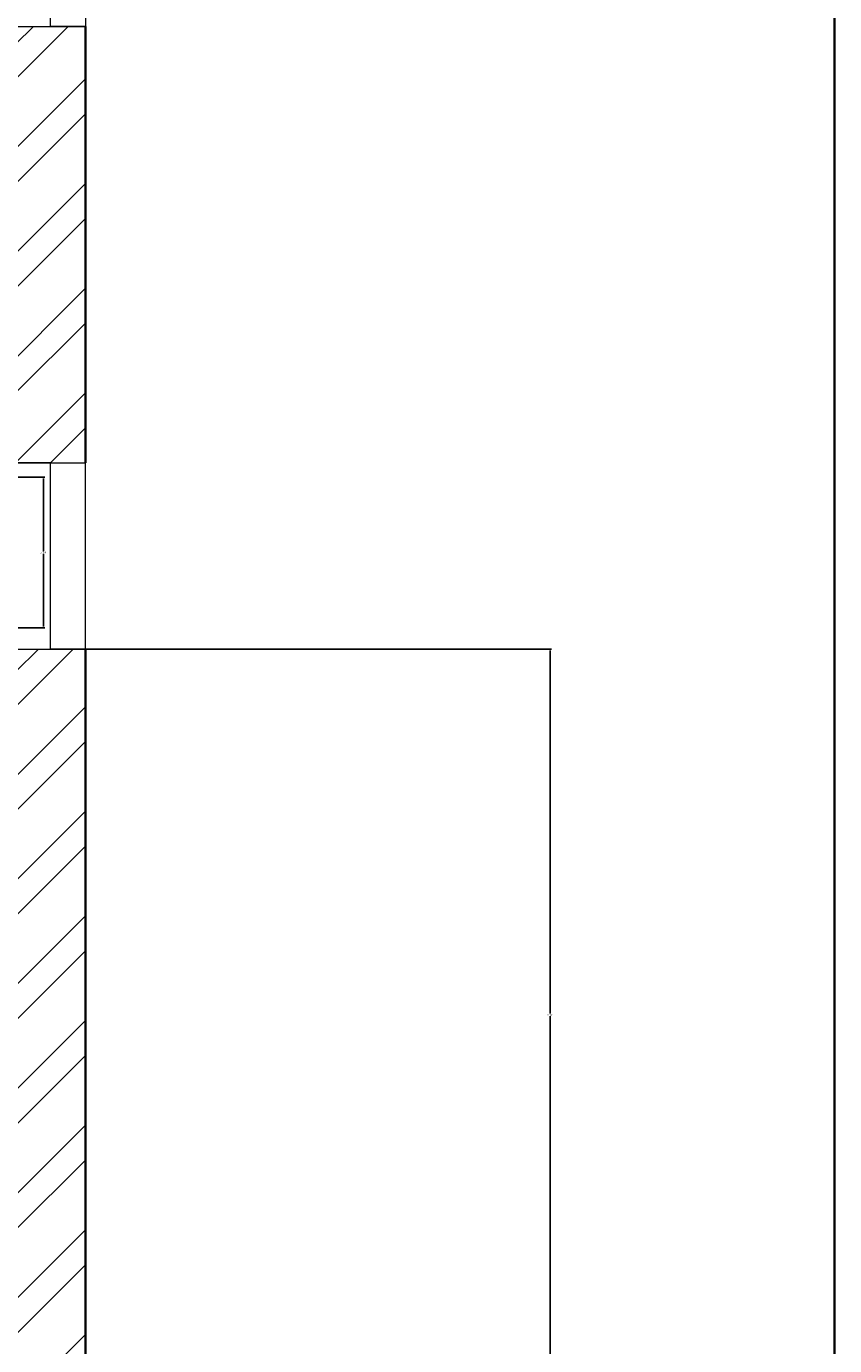
# Model space of a CAD drawing. Units: inches. Extents: x 2552 to 3217, y 1417 to 2737.
# Tile 24 of 25: x 3113 to 3217, y 2392 to 2561. Entities that reach past the tile are written whole.
import ezdxf

# ---------------------------------------------------------------- set-up
doc = ezdxf.new("R2010")
doc.units = ezdxf.units.IN
for name, color, linetype, lineweight in [('A-ANNO-DIMS', 2, 'Continuous', 18), ('A-ANNO-TTLB', 7, 'Continuous', 35), ('A-GLAZ', 161, 'Continuous', 18), ('A-WALL', 7, 'Continuous', 35), ('A-WALL-PATT', 217, 'Continuous', 13)]:
    doc.layers.add(name, color=color, linetype=linetype, lineweight=lineweight)
doc.styles.get("Standard").update_dxf_attribs({"font": 'arial.ttf'})
doc.dimstyles.get("Standard").update_dxf_attribs({"dimtxt": 0.18, "dimasz": 0.18, "dimexe": 0.18, "dimexo": 0.0625, "dimgap": 0.09, "dimtad": 0, "dimtih": 1, "dimtoh": 1, "dimdec": 4, "dimzin": 0, "dimdsep": 46, "dimtxsty": 'Standard', "dimcen": 0.09, "dimadec": 0, "dimazin": 0, "dimtfac": 1, "dimtdec": 4, "dimtofl": 0, "dimtmove": 0, "dimatfit": 3, "dimfxl": 1, "dimtolj": 1, "dimtzin": 0, "dimarcsym": 0})

# ---------------------------------------------------------------- blocks, each defined once
blk = doc.blocks.new('WIN-48')
for p, q in [((4.5, 48), (0, 48)), ((0, 48), (9, 48)), ((0, 48), (0, 0)), ((4.5, 0), (4.5, 48)), ((9, 48), (9, 0)), ((0, 0), (9, 0)), ((9, 0), (4.5, 0))]:
    blk.add_line(p, q)
blk = doc.blocks.new('WIN-24')
for p, q in [((0, 24), (9, 24)), ((0, 24), (0, 0)), ((9, 24), (4.5, 24)), ((4.5, 24), (4.5, 0)), ((9, 24), (9, 0)), ((4.5, 0), (0, 0)), ((0, 0), (9, 0))]:
    blk.add_line(p, q)
blk = doc.blocks.new('*D18')
at = {"layer": 'A-ANNO-DIMS', "color": 0, "lineweight": -2, "transparency": 16777216}
for p, q in [((3110.68, 2503.32), (3115.11, 2503.32)), ((3114.93, 2503.14), (3114.93, 2493.81)), ((3114.93, 2484.12), (3114.93, 2493.45)), ((3110.68, 2483.94), (3115.11, 2483.94))]:
    blk.add_line(p, q, dxfattribs=at)
at = {"layer": 'A-ANNO-DIMS', "color": 0, "transparency": 16777216}
for points in [[(3114.9, 2503.14), (3114.96, 2503.14), (3114.93, 2503.32)], [(3114.9, 2484.12), (3114.96, 2484.12), (3114.93, 2483.94)]]:
    blk.add_solid(points, dxfattribs=at)
at = {"layer": 'Defpoints', "color": 0, "transparency": 16777216}
for p in [(3110.62, 2503.32), (3114.93, 2503.32), (3110.62, 2483.94)]:
    blk.add_point(p, dxfattribs=at)
at = {"layer": 'A-ANNO-DIMS', "color": 0, "transparency": 16777216, "insert": (3114.93, 2493.63), "char_height": 0.18, "attachment_point": 5}
blk.add_mtext('\\A1;19 TYP.', dxfattribs=at)
blk = doc.blocks.new('*D66')
at = {"layer": 'A-ANNO-DIMS', "color": 0, "lineweight": -2, "transparency": 16777216}
for p, q in [((3120.42, 2481.18), (3180.33, 2481.18)), ((3180.15, 2481), (3180.15, 2434.28)), ((3180.15, 2387.19), (3180.15, 2433.92)), ((3111.42, 2387.01), (3180.33, 2387.01))]:
    blk.add_line(p, q, dxfattribs=at)
at = {"layer": 'A-ANNO-DIMS', "color": 0, "transparency": 16777216}
for points in [[(3180.12, 2481), (3180.18, 2481), (3180.15, 2481.18)], [(3180.12, 2387.19), (3180.18, 2387.19), (3180.15, 2387.01)]]:
    blk.add_solid(points, dxfattribs=at)
at = {"layer": 'Defpoints', "color": 0, "transparency": 16777216}
for p in [(3120.35, 2481.18), (3111.35, 2387.01), (3180.15, 2387.01)]:
    blk.add_point(p, dxfattribs=at)
at = {"layer": 'A-ANNO-DIMS', "color": 0, "transparency": 16777216, "insert": (3180.15, 2434.1), "char_height": 0.18, "attachment_point": 5}
blk.add_mtext('\\A1;94.17', dxfattribs=at)

msp = doc.modelspace()

# ---------------------------------------------------------------- hatches: boundary and pattern name
at = {"layer": 'A-WALL-PATT'}
h = msp.add_hatch(dxfattribs=at)
h.set_pattern_fill('ANSI32', color=256)
h.paths.add_polyline_path([(2756.676, 2649.5125), (2637.3535, 2649.5125), (2637.3535, 2617.9626), (2641.8535, 2617.9626), (2646.3535, 2617.9626), (2646.3535, 2640.5125), (2724.3535, 2640.5125), (2724.3535, 2520.5125), (2720.299, 2520.5125), (2720.299, 2516.0125), (2733.4075, 2516.0125), (2733.4075, 2518.2213), (2733.4075, 2520.5125), (2728.8535, 2520.5125), (2728.8535, 2640.5125), (2756.676, 2640.5125)])
h.paths.add_polyline_path([(2848.8535, 2649.5125), (2804.676, 2649.5125), (2804.676, 2640.5125), (2839.8535, 2640.5125), (2839.8535, 2598.3517), (2848.8535, 2598.3517)])
h.paths.add_polyline_path([(2646.3535, 2516.0125), (2697.9593, 2516.0125), (2697.9593, 2518.2625), (2697.9593, 2520.5125), (2646.3535, 2520.5125), (2646.3535, 2581.9626), (2637.3535, 2581.9626), (2637.3535, 2364.3298), (2646.3535, 2364.3298), (2646.3535, 2387.0125), (2724.3535, 2387.0125), (2724.3535, 2267.0125), (2721.0443, 2267.0125), (2721.0443, 2262.5125), (2733.7854, 2262.5125), (2733.7854, 2264.7625), (2733.7854, 2267.0125), (2728.8535, 2267.0125), (2728.8535, 2387.0125), (2839.8535, 2387.0125), (2839.8535, 2363.8387), (2848.8535, 2363.8387), (2848.8535, 2403.7415), (2844.3535, 2403.7415), (2839.8535, 2403.7415), (2839.8535, 2396.0125), (2646.3535, 2396.0125)])
h.paths.add_polyline_path([(2848.8535, 2550.3517), (2844.3535, 2550.3517), (2839.8535, 2550.3517), (2839.8535, 2520.5125), (2801.9195, 2520.5125), (2801.9195, 2518.2625), (2801.9195, 2516.0125), (2839.8535, 2516.0125), (2839.8535, 2507.5813), (2848.8535, 2507.5813)], flags=17)
h.paths.add_polyline_path([(2848.8535, 2483.5813), (2844.3535, 2483.5813), (2839.8535, 2483.5813), (2839.8535, 2468.0125), (2773.8535, 2468.0125), (2773.8535, 2516.0125), (2778.1336, 2516.0125), (2778.1336, 2520.5125), (2766.696, 2520.5125), (2766.696, 2518.2625), (2766.696, 2516.0125), (2769.3535, 2516.0125), (2769.3535, 2463.5125), (2839.8535, 2463.5125), (2839.8535, 2431.0782), (2848.8535, 2431.0782)], flags=17)
h.paths.add_polyline_path([(2917.8535, 2569.2764), (2913.3535, 2569.2764), (2908.8535, 2569.2764), (2908.8535, 2433.001), (2917.8535, 2433.001), (2917.8535, 2516.0125), (2967.486, 2516.0125), (2967.486, 2520.5125), (2917.8535, 2520.5125)])
h.paths.add_polyline_path([(3000.3535, 2640.5125), (2995.8535, 2640.5125), (2995.8535, 2520.5125), (2990.688, 2520.5125), (2990.688, 2516.0125), (3004.0844, 2516.0125), (3004.0844, 2518.2625), (3004.0844, 2520.5125), (3000.3535, 2520.5125)])
h.paths.add_polyline_path([(3120.3535, 2561.3689), (3115.8535, 2561.3689), (3111.3535, 2561.3689), (3111.3535, 2520.5125), (3070.9814, 2520.5125), (3070.9814, 2518.2625), (3070.9814, 2516.0125), (3111.3535, 2516.0125), (3111.3535, 2505.1841), (3120.3535, 2505.1841)])
h.paths.add_polyline_path([(3120.3535, 2481.1841), (3115.8535, 2481.1841), (3111.3535, 2481.1841), (3111.3535, 2468.0125), (3045.3535, 2468.0125), (3045.3535, 2516.0125), (3048.9787, 2516.0125), (3048.9787, 2520.5125), (3036.3395, 2520.5125), (3036.3395, 2516.0125), (3040.8535, 2516.0125), (3040.8535, 2463.5125), (3111.3535, 2463.5125), (3111.3535, 2396.0125), (2917.8535, 2396.0125), (2917.8535, 2403.4124), (2913.3535, 2403.4124), (2908.8535, 2403.4124), (2908.8535, 2182.5756), (2917.8535, 2182.5756), (2917.8535, 2262.5125), (2968.001, 2262.5125), (2968.001, 2264.7625), (2968.001, 2267.0125), (2917.8535, 2267.0125), (2917.8535, 2387.0125), (3111.3535, 2387.0125), (3111.3535, 2352.2435), (3120.3535, 2352.2435)])
h.paths.add_polyline_path([(3120.3535, 2304.2435), (3115.8535, 2304.2435), (3111.3535, 2304.2435), (3111.3535, 2267.0125), (3073.8616, 2267.0125), (3073.8616, 2264.7625), (3073.8616, 2262.5125), (3111.3535, 2262.5125), (3111.3535, 2252.376), (3120.3535, 2252.376)], flags=17)
h.paths.add_polyline_path([(3120.3535, 2228.376), (3115.8535, 2228.376), (3111.3535, 2228.376), (3111.3535, 2214.5125), (3045.3535, 2214.5125), (3045.3535, 2262.5125), (3049.3096, 2262.5125), (3049.3096, 2267.0125), (3035.0125, 2267.0125), (3035.0125, 2262.5125), (3040.8535, 2262.5125), (3040.8535, 2210.0125), (3111.3535, 2210.0125), (3111.3535, 2142.5125), (2917.8535, 2142.5125), (2917.8535, 2150.2408), (2913.3535, 2150.2408), (2908.8535, 2150.2408), (2908.8535, 1924.9905), (2917.8535, 1924.9905), (2917.8535, 2009.0125), (2971.959, 2009.0125), (2971.959, 2011.2625), (2971.959, 2013.5125), (2917.8535, 2013.5125), (2917.8535, 2133.5125), (2995.8535, 2133.5125), (2995.8535, 2013.5125), (2992.1797, 2013.5125), (2992.1797, 2009.0125), (3004.3344, 2009.0125), (3004.3344, 2011.2625), (3004.3344, 2013.5125), (3000.3535, 2013.5125), (3000.3535, 2133.5125), (3111.3535, 2133.5125), (3111.3535, 2115.0291), (3120.3535, 2115.0291)])
h.paths.add_polyline_path([(3000.3535, 2387.0125), (2995.8535, 2387.0125), (2995.8535, 2267.0125), (2991.3326, 2267.0125), (2991.3326, 2262.5125), (3004.1044, 2262.5125), (3004.1044, 2264.7625), (3004.1044, 2267.0125), (3000.3535, 2267.0125)], flags=17)
h.paths.add_polyline_path([(3120.3535, 1973.2388), (3115.8535, 1973.2388), (3111.3535, 1973.2388), (3111.3535, 1961.0125), (3045.3535, 1961.0125), (3045.3535, 2009.0125), (3048.9101, 2009.0125), (3048.9101, 2013.5125), (3037.105, 2013.5125), (3037.105, 2011.2625), (3037.105, 2009.0125), (3040.8535, 2009.0125), (3040.8535, 1956.5125), (3111.3535, 1956.5125), (3111.3535, 1889.0125), (2917.8535, 1889.0125), (2917.8535, 1895.7215), (2913.3535, 1895.7215), (2908.8535, 1895.7215), (2908.8535, 1844.2217), (2917.8535, 1844.2217), (2917.8535, 1880.0125), (3111.3535, 1880.0125), (3111.3535, 1846.9541), (3120.3535, 1846.9541)])
h.paths.add_polyline_path([(3120.3535, 2067.0291), (3111.3535, 2067.0291), (3111.3535, 2013.5125), (3071.3001, 2013.5125), (3071.3001, 2009.0125), (3111.3535, 2009.0125), (3111.3535, 1997.2388), (3120.3535, 1997.2388)], flags=0)
h.paths.add_polyline_path([(3120.3535, 1798.9541), (3115.8535, 1798.9541), (3111.3535, 1798.9541), (3111.3535, 1760.0125), (3071.2497, 1760.0125), (3071.2497, 1757.7625), (3071.2497, 1755.5125), (3111.3535, 1755.5125), (3111.3535, 1746.162), (3120.3535, 1746.2478)])
h.paths.add_polyline_path([(3120.3535, 1722.2049), (3111.3535, 1722.2049), (3111.3535, 1707.5125), (3045.3535, 1707.5125), (3045.3535, 1755.5125), (3048.6624, 1755.5125), (3048.6624, 1760.0125), (3035.3703, 1760.0125), (3035.3703, 1755.5125), (3040.8535, 1755.5125), (3040.8535, 1703.0125), (3111.3535, 1703.0125), (3111.3535, 1635.5125), (2917.8535, 1635.5125), (2917.8535, 1643.1366), (2913.3535, 1643.1366), (2908.8535, 1643.1366), (2908.8535, 1626.5125), (3120.3535, 1626.5125)])
h.paths.add_polyline_path([(2917.8535, 1755.5125), (2973.2287, 1755.5125), (2973.2287, 1757.7625), (2973.2287, 1760.0125), (2917.8535, 1760.0125), (2917.8535, 1808.2217), (2913.3535, 1808.2217), (2908.8535, 1808.2217), (2908.8535, 1676.1665), (2917.8535, 1676.1665)])
h.paths.add_polyline_path([(3000.3535, 1880.0125), (2995.8535, 1880.0125), (2995.8535, 1760.0125), (2992.9329, 1760.0125), (2992.9329, 1755.5125), (3003.8766, 1755.5125), (3003.8766, 1757.7625), (3003.8766, 1760.0125), (3000.3535, 1760.0125)])
h.paths.add_polyline_path([(2848.8535, 1896.6971), (2844.3535, 1896.6971), (2839.8535, 1896.6971), (2839.8535, 1889.0125), (2646.3535, 1889.0125), (2646.3535, 2009.0125), (2700.5253, 2009.0125), (2700.5253, 2011.2625), (2700.5253, 2013.5125), (2646.3535, 2013.5125), (2646.3535, 2053.1812), (2641.8535, 2053.1812), (2637.3535, 2053.1812), (2637.3535, 1836.254), (2646.3535, 1836.254), (2646.3535, 1880.0125), (2724.3535, 1880.0125), (2724.3535, 1760.0125), (2721.2473, 1760.0125), (2721.2473, 1755.5125), (2731.9187, 1755.5125), (2731.9187, 1757.7625), (2731.9187, 1760.0125), (2728.8535, 1760.0125), (2728.8535, 1880.0125), (2839.8535, 1880.0125), (2839.8535, 1840.3813), (2848.8535, 1840.3813)])
h.paths.add_polyline_path([(2848.8535, 1792.3813), (2844.3535, 1792.3813), (2839.8535, 1792.3813), (2839.8535, 1760.0125), (2797.8845, 1760.0125), (2797.8845, 1755.5125), (2839.8535, 1755.5125), (2839.8535, 1743.3688), (2844.3535, 1743.3688), (2848.8535, 1743.3688)], flags=0)
h.paths.add_polyline_path([(2848.8535, 1719.3688), (2844.3535, 1719.3688), (2839.8535, 1719.3688), (2839.8535, 1707.5125), (2773.8535, 1707.5125), (2773.8535, 1755.5125), (2777.716, 1755.5125), (2777.716, 1760.0125), (2760.9247, 1760.0125), (2760.9247, 1757.9721), (2760.9247, 1755.5125), (2769.3535, 1755.5125), (2769.3535, 1703.0125), (2839.8535, 1703.0125), (2839.8535, 1673.0277), (2848.8535, 1672.9407)], flags=0)
h.paths.add_polyline_path([(2646.3535, 1755.5125), (2702.9171, 1755.5125), (2702.9171, 1757.7625), (2702.9171, 1760.0125), (2646.3535, 1760.0125), (2646.3535, 1800.254), (2641.8535, 1800.254), (2637.3535, 1800.254), (2637.3535, 1626.5125), (2848.8535, 1626.5125), (2848.8535, 1643.1187), (2844.3535, 1643.1187), (2839.8535, 1643.1187), (2839.8535, 1635.5125), (2646.3535, 1635.5125)])
h.paths.add_polyline_path([(2848.8535, 2148.8427), (2844.3535, 2148.8427), (2839.8535, 2148.8427), (2839.8535, 2142.5125), (2646.3535, 2142.5125), (2646.3535, 2262.5125), (2701.3562, 2262.5125), (2701.3562, 2264.7625), (2701.3562, 2267.0125), (2646.3535, 2267.0125), (2646.3535, 2328.3298), (2637.3535, 2328.3298), (2637.3535, 2089.1812), (2646.3535, 2089.1812), (2646.3535, 2133.5125), (2839.8535, 2133.5125), (2839.8535, 2097.5966), (2848.8535, 2097.5966)])
h.paths.add_polyline_path([(2728.8535, 2133.5125), (2724.3535, 2133.5125), (2724.3535, 2013.5125), (2719.6039, 2013.5125), (2719.6039, 2009.0125), (2732.5784, 2009.0125), (2732.5784, 2011.2625), (2732.5784, 2013.5125), (2728.8535, 2013.5125)])
h.paths.add_polyline_path([(2848.8535, 1970.0557), (2844.3535, 1970.0557), (2839.8535, 1970.0557), (2839.8535, 1961.0125), (2773.8535, 1961.0125), (2773.8535, 2009.0125), (2777.3388, 2009.0125), (2777.3388, 2013.5125), (2764.7681, 2013.5125), (2764.7681, 2009.0125), (2769.3535, 2009.0125), (2769.3535, 1956.5125), (2839.8535, 1956.5125), (2839.8535, 1924.7199), (2848.8535, 1924.7199)], flags=17)
h.paths.add_polyline_path([(2848.8535, 2049.5966), (2844.3535, 2049.5966), (2839.8535, 2049.5966), (2839.8535, 2013.5125), (2798.198, 2013.5125), (2798.198, 2011.2625), (2798.198, 2009.0125), (2839.8535, 2009.0125), (2839.8535, 1994.0557), (2848.8535, 1994.0557)], flags=17)
h.paths.add_polyline_path([(2848.8535, 2315.8387), (2839.8535, 2315.8387), (2839.8535, 2267.0125), (2799.3375, 2267.0125), (2799.3375, 2264.7625), (2799.3375, 2262.5125), (2839.8535, 2262.5125), (2839.8535, 2253.2843), (2848.8535, 2253.2843)], flags=17)
h.paths.add_polyline_path([(2848.8535, 2229.2843), (2839.8535, 2229.2843), (2839.8535, 2177.6936), (2848.8535, 2177.6936)], flags=17)
h.paths.add_polyline_path([(2839.8535, 2214.5125), (2773.8535, 2214.5125), (2773.8535, 2262.5125), (2777.6984, 2262.5125), (2777.6984, 2267.0125), (2763.8226, 2267.0125), (2763.8226, 2262.5125), (2769.3535, 2262.5125), (2769.3535, 2210.0125), (2839.8535, 2210.0125)], flags=17)
h.paths.add_polyline_path([(3050.32, 2520.2817), (3088.9114, 2520.2817), (3088.9114, 2538.939), (3050.32, 2538.939)], flags=9)

# ---------------------------------------------------------------- linework, layer by layer
at = {"layer": 'A-ANNO-TTLB'}
msp.add_lwpolyline([(2552.473, 2736.5692), (3216.7862, 2736.5692), (3216.7862, 1416.6914), (2552.473, 1416.6914)], close=True, dxfattribs=at)
at = {"layer": 'A-GLAZ'}
msp.add_line((3115.8535, 2481.1841), (3115.8535, 2481.1841), dxfattribs=at)
at = {"layer": 'A-WALL'}
for p, q in [((3120.3535, 2561.3689), (3120.3535, 2505.1841)), ((3120.3535, 2481.1841), (3120.3535, 2352.2435))]:
    msp.add_line(p, q, dxfattribs=at)

# ---------------------------------------------------------------- block references
at = {"layer": 'A-GLAZ'}
msp.add_blockref('WIN-48', (3111.354, 2561.3694), dxfattribs=at)
at = {"layer": 'A-GLAZ', "extrusion": (0, 0, -1), "zscale": -1, "rotation": 180}
msp.add_blockref('WIN-24', (-3111.354, 2505.1844), dxfattribs=at)

# ---------------------------------------------------------------- dimensions: what is measured, and where the dimension line sits
at = {"layer": 'A-ANNO-DIMS'}
dim = msp.add_linear_dim(base=(3114.9275, 2503.3228), p1=(3110.6194, 2483.9415), p2=(3110.6194, 2503.3228), angle=90, text='<> TYP.', dimstyle='Standard', override={"dimdec": 0, "dimlfac": 1, "dimrnd": 0, "dimzin": 0, "dimdsep": 46, "dimlunit": 2}, dxfattribs=at)
dim.commit()
dim.dimension.update_dxf_attribs({"geometry": '*D18', "text_midpoint": (3114.9275, 2493.6322)})
dim = msp.add_linear_dim(base=(3180.1535, 2387.0125), p1=(3120.3535, 2481.1841), p2=(3111.3535, 2387.0125), angle=90, dimstyle='Standard', override={"dimdec": 2, "dimlfac": 1, "dimrnd": 0, "dimzin": 0, "dimdsep": 46, "dimlunit": 2}, dxfattribs=at)
dim.commit()
dim.dimension.update_dxf_attribs({"geometry": '*D66', "text_midpoint": (3180.1535, 2434.0983)})

doc.saveas('drawing.dxf')
